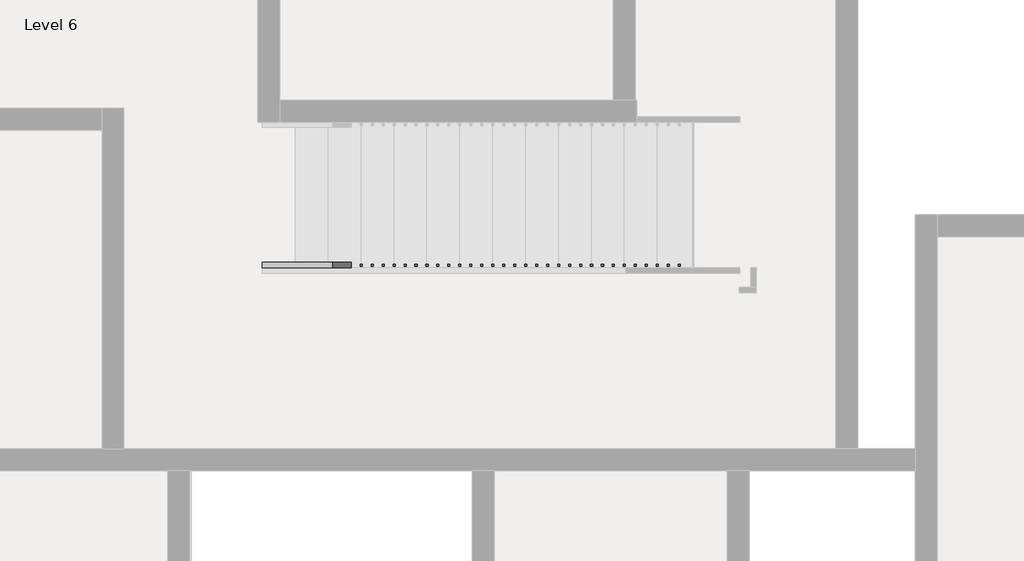
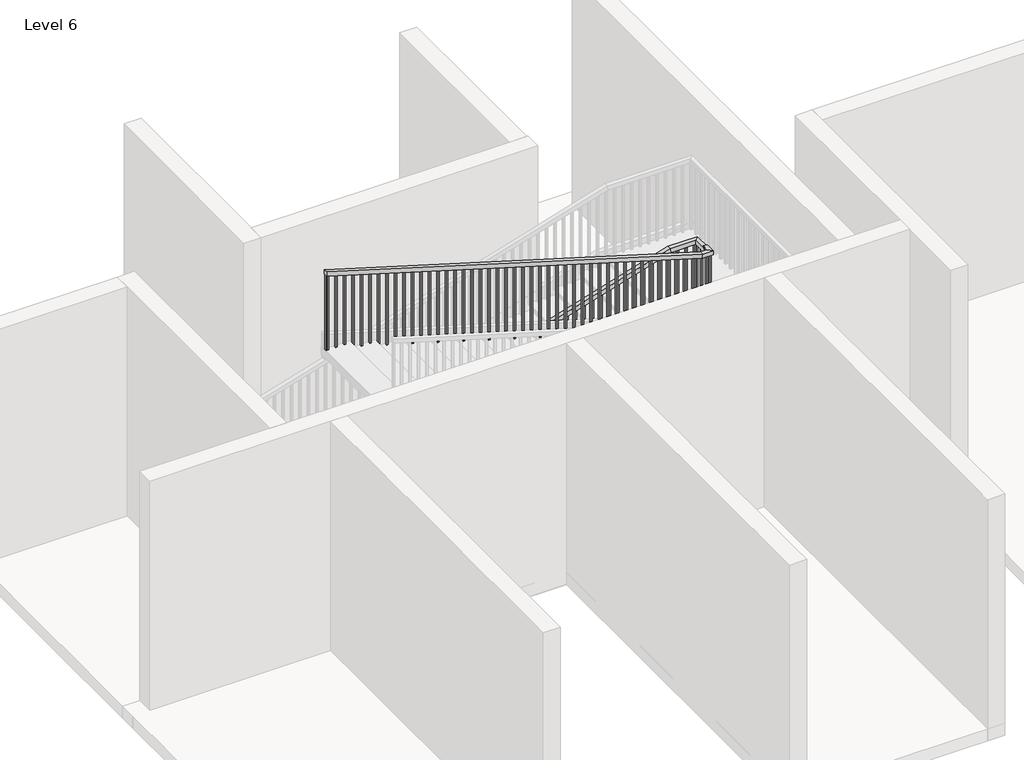
# One storey, part 11 of 14: 1 railing.
"""IFC4 building model written with IfcOpenShell, lengths in millimetres."""

from ifc_helpers import new_model, si_unit, frame, origin, place, context, project, spatial, polyline, outline, extrude, faceted_brep, element, save

model = new_model("IFC4")

# Units and contexts
model_context = context("Model", 3, world=origin())
ifc_project = project(units=[si_unit("LENGTHUNIT", "METRE", prefix="MILLI")], contexts=[model_context])

# Site, building, storey
site = spatial("IfcSite", under=ifc_project)
building = spatial("IfcBuilding", under=site)
storey = spatial("IfcBuildingStorey", under=building, Name="Level 6", Elevation=15240.0)

# Railing
placement = place(None, origin())
element("IfcRailing", 1, ObjectType="Handrail - Rectangular", at=placement, inside=storey, context=model_context, shape_type="SolidModel", body=[
    faceted_brep([(-5254.0891351, 11205.0082924, 16245.84), (-5254.0891351, 11205.0082924, 16192.8032429), (-5254.0891351, 11154.2082924, 16192.8032429), (-5254.0891351, 11154.2082924, 16245.84), (-986.8891351, 11205.0082924, 17526.0), (-979.4332782, 11205.0082924, 17475.2), (-979.4332782, 11154.2082924, 17475.2), (-986.8891351, 11154.2082924, 17526.0), (-631.2891351, 11205.0082924, 17526.0), (-631.2891351, 11205.0082924, 17475.2), (-682.0891351, 11154.2082924, 17475.2), (-682.0891351, 11154.2082924, 17526.0), (-631.2891351, 11001.8082924, 17526.0), (-631.2891351, 10951.0082924, 17475.2), (-682.0891351, 10951.0082924, 17475.2), (-682.0891351, 11001.8082924, 17526.0), (-631.2891351, 11001.8082924, 17548.86), (-631.2891351, 10951.0082924, 17498.06), (-682.0891351, 10951.0082924, 17498.06), (-682.0891351, 11001.8082924, 17548.86), (-631.2891351, 10874.8082924, 17548.86), (-631.2891351, 10874.8082924, 17498.06), (-682.0891351, 10925.6082924, 17498.06), (-682.0891351, 10925.6082924, 17548.86), (-758.2891351, 10874.8082924, 17548.86), (-765.744992, 10874.8082924, 17498.06), (-765.744992, 10925.6082924, 17498.06), (-758.2891351, 10925.6082924, 17548.86), (-5254.0891351, 10874.8082924, 18897.6), (-5254.0891351, 10925.6082924, 18897.6), (-5254.0891351, 10925.6082924, 18844.5632429), (-5254.0891351, 10874.8082924, 18844.5632429)], [[[0, 1, 2, 3]], [[1, 0, 4, 5]], [[2, 1, 5, 6]], [[3, 2, 6, 7]], [[0, 3, 7, 4]], [[5, 4, 8, 9]], [[6, 5, 9, 10]], [[7, 6, 10, 11]], [[4, 7, 11, 8]], [[9, 8, 12, 13]], [[10, 9, 13, 14]], [[11, 10, 14, 15]], [[8, 11, 15, 12]], [[13, 12, 16, 17]], [[14, 13, 17, 18]], [[15, 14, 18, 19]], [[12, 15, 19, 16]], [[17, 16, 20, 21]], [[18, 17, 21, 22]], [[19, 18, 22, 23]], [[16, 19, 23, 20]], [[21, 20, 24, 25]], [[22, 21, 25, 26]], [[23, 22, 26, 27]], [[20, 23, 27, 24]], [[28, 29, 30, 31]], [[25, 24, 28, 31]], [[26, 25, 31, 30]], [[27, 26, 30, 29]], [[24, 27, 29, 28]]]),
    extrude(outline(polyline([(18834.0857429, -5219.1641351), (18839.8007429, -5238.2141351), (17891.76, -5238.2141351), (17891.76, -5219.1641351), (18834.0857429, -5219.1641351)])), frame((0.0, 10890.6832924, 0.0), z_axis=(0.0, 1.0, 0.0), x_axis=(0.0, 0.0, 1.0)), (0.0, 0.0, 1.0), 19.05),
    extrude(outline(polyline([(18803.6057429, -5117.5641351), (18809.3207429, -5136.6141351), (17891.76, -5136.6141351), (17891.76, -5117.5641351), (18803.6057429, -5117.5641351)])), frame((0.0, 10890.6832924, 0.0), z_axis=(0.0, 1.0, 0.0), x_axis=(0.0, 0.0, 1.0)), (0.0, 0.0, 1.0), 19.05),
    extrude(outline(polyline([(18773.1257429, -5015.9641351), (18778.8407429, -5035.0141351), (17891.76, -5035.0141351), (17891.76, -5015.9641351), (18773.1257429, -5015.9641351)])), frame((0.0, 10890.6832924, 0.0), z_axis=(0.0, 1.0, 0.0), x_axis=(0.0, 0.0, 1.0)), (0.0, 0.0, 1.0), 19.05),
    extrude(outline(polyline([(18742.6457429, -4914.3641351), (18748.3607429, -4933.4141351), (17800.32, -4933.4141351), (17800.32, -4914.3641351), (18742.6457429, -4914.3641351)])), frame((0.0, 10890.6832924, 0.0), z_axis=(0.0, 1.0, 0.0), x_axis=(0.0, 0.0, 1.0)), (0.0, 0.0, 1.0), 19.05),
    extrude(outline(polyline([(18712.1657429, -4812.7641351), (18717.8807429, -4831.8141351), (17800.32, -4831.8141351), (17800.32, -4812.7641351), (18712.1657429, -4812.7641351)])), frame((0.0, 10890.6832924, 0.0), z_axis=(0.0, 1.0, 0.0), x_axis=(0.0, 0.0, 1.0)), (0.0, 0.0, 1.0), 19.05),
    extrude(outline(polyline([(18681.6857429, -4711.1641351), (18687.4007429, -4730.2141351), (17800.32, -4730.2141351), (17800.32, -4711.1641351), (18681.6857429, -4711.1641351)])), frame((0.0, 10890.6832924, 0.0), z_axis=(0.0, 1.0, 0.0), x_axis=(0.0, 0.0, 1.0)), (0.0, 0.0, 1.0), 19.05),
    extrude(outline(polyline([(18651.2057429, -4609.5641351), (18656.9207429, -4628.6141351), (17708.88, -4628.6141351), (17708.88, -4609.5641351), (18651.2057429, -4609.5641351)])), frame((0.0, 10890.6832924, 0.0), z_axis=(0.0, 1.0, 0.0), x_axis=(0.0, 0.0, 1.0)), (0.0, 0.0, 1.0), 19.05),
    extrude(outline(polyline([(18620.7257429, -4507.9641351), (18626.4407429, -4527.0141351), (17708.88, -4527.0141351), (17708.88, -4507.9641351), (18620.7257429, -4507.9641351)])), frame((0.0, 10890.6832924, 0.0), z_axis=(0.0, 1.0, 0.0), x_axis=(0.0, 0.0, 1.0)), (0.0, 0.0, 1.0), 19.05),
    extrude(outline(polyline([(18590.2457429, -4406.3641351), (18595.9607429, -4425.4141351), (17708.88, -4425.4141351), (17708.88, -4406.3641351), (18590.2457429, -4406.3641351)])), frame((0.0, 10890.6832924, 0.0), z_axis=(0.0, 1.0, 0.0), x_axis=(0.0, 0.0, 1.0)), (0.0, 0.0, 1.0), 19.05),
    extrude(outline(polyline([(18559.7657429, -4304.7641351), (18565.4807429, -4323.8141351), (17617.44, -4323.8141351), (17617.44, -4304.7641351), (18559.7657429, -4304.7641351)])), frame((0.0, 10890.6832924, 0.0), z_axis=(0.0, 1.0, 0.0), x_axis=(0.0, 0.0, 1.0)), (0.0, 0.0, 1.0), 19.05),
    extrude(outline(polyline([(18529.2857429, -4203.1641351), (18535.0007429, -4222.2141351), (17617.44, -4222.2141351), (17617.44, -4203.1641351), (18529.2857429, -4203.1641351)])), frame((0.0, 10890.6832924, 0.0), z_axis=(0.0, 1.0, 0.0), x_axis=(0.0, 0.0, 1.0)), (0.0, 0.0, 1.0), 19.05),
    extrude(outline(polyline([(18498.8057429, -4101.5641351), (18504.5207429, -4120.6141351), (17617.44, -4120.6141351), (17617.44, -4101.5641351), (18498.8057429, -4101.5641351)])), frame((0.0, 10890.6832924, 0.0), z_axis=(0.0, 1.0, 0.0), x_axis=(0.0, 0.0, 1.0)), (0.0, 0.0, 1.0), 19.05),
    extrude(outline(polyline([(18468.3257429, -3999.9641351), (18474.0407429, -4019.0141351), (17526.0, -4019.0141351), (17526.0, -3999.9641351), (18468.3257429, -3999.9641351)])), frame((0.0, 10890.6832924, 0.0), z_axis=(0.0, 1.0, 0.0), x_axis=(0.0, 0.0, 1.0)), (0.0, 0.0, 1.0), 19.05),
    extrude(outline(polyline([(18437.8457429, -3898.3641351), (18443.5607429, -3917.4141351), (17526.0, -3917.4141351), (17526.0, -3898.3641351), (18437.8457429, -3898.3641351)])), frame((0.0, 10890.6832924, 0.0), z_axis=(0.0, 1.0, 0.0), x_axis=(0.0, 0.0, 1.0)), (0.0, 0.0, 1.0), 19.05),
    extrude(outline(polyline([(18407.3657429, -3796.7641351), (18413.0807429, -3815.8141351), (17526.0, -3815.8141351), (17526.0, -3796.7641351), (18407.3657429, -3796.7641351)])), frame((0.0, 10890.6832924, 0.0), z_axis=(0.0, 1.0, 0.0), x_axis=(0.0, 0.0, 1.0)), (0.0, 0.0, 1.0), 19.05),
    extrude(outline(polyline([(18376.8857429, -3695.1641351), (18382.6007429, -3714.2141351), (17434.56, -3714.2141351), (17434.56, -3695.1641351), (18376.8857429, -3695.1641351)])), frame((0.0, 10890.6832924, 0.0), z_axis=(0.0, 1.0, 0.0), x_axis=(0.0, 0.0, 1.0)), (0.0, 0.0, 1.0), 19.05),
    extrude(outline(polyline([(18346.4057429, -3593.5641351), (18352.1207429, -3612.6141351), (17434.56, -3612.6141351), (17434.56, -3593.5641351), (18346.4057429, -3593.5641351)])), frame((0.0, 10890.6832924, 0.0), z_axis=(0.0, 1.0, 0.0), x_axis=(0.0, 0.0, 1.0)), (0.0, 0.0, 1.0), 19.05),
    extrude(outline(polyline([(18315.9257429, -3491.9641351), (18321.6407429, -3511.0141351), (17434.56, -3511.0141351), (17434.56, -3491.9641351), (18315.9257429, -3491.9641351)])), frame((0.0, 10890.6832924, 0.0), z_axis=(0.0, 1.0, 0.0), x_axis=(0.0, 0.0, 1.0)), (0.0, 0.0, 1.0), 19.05),
    extrude(outline(polyline([(18285.4457429, -3390.3641351), (18291.1607429, -3409.4141351), (17343.12, -3409.4141351), (17343.12, -3390.3641351), (18285.4457429, -3390.3641351)])), frame((0.0, 10890.6832924, 0.0), z_axis=(0.0, 1.0, 0.0), x_axis=(0.0, 0.0, 1.0)), (0.0, 0.0, 1.0), 19.05),
    extrude(outline(polyline([(18254.9657429, -3288.7641351), (18260.6807429, -3307.8141351), (17343.12, -3307.8141351), (17343.12, -3288.7641351), (18254.9657429, -3288.7641351)])), frame((0.0, 10890.6832924, 0.0), z_axis=(0.0, 1.0, 0.0), x_axis=(0.0, 0.0, 1.0)), (0.0, 0.0, 1.0), 19.05),
    extrude(outline(polyline([(18224.4857429, -3187.1641351), (18230.2007429, -3206.2141351), (17343.12, -3206.2141351), (17343.12, -3187.1641351), (18224.4857429, -3187.1641351)])), frame((0.0, 10890.6832924, 0.0), z_axis=(0.0, 1.0, 0.0), x_axis=(0.0, 0.0, 1.0)), (0.0, 0.0, 1.0), 19.05),
    extrude(outline(polyline([(18194.0057429, -3085.5641351), (18199.7207429, -3104.6141351), (17251.68, -3104.6141351), (17251.68, -3085.5641351), (18194.0057429, -3085.5641351)])), frame((0.0, 10890.6832924, 0.0), z_axis=(0.0, 1.0, 0.0), x_axis=(0.0, 0.0, 1.0)), (0.0, 0.0, 1.0), 19.05),
    extrude(outline(polyline([(18163.5257429, -2983.9641351), (18169.2407429, -3003.0141351), (17251.68, -3003.0141351), (17251.68, -2983.9641351), (18163.5257429, -2983.9641351)])), frame((0.0, 10890.6832924, 0.0), z_axis=(0.0, 1.0, 0.0), x_axis=(0.0, 0.0, 1.0)), (0.0, 0.0, 1.0), 19.05),
    extrude(outline(polyline([(18133.0457429, -2882.3641351), (18138.7607429, -2901.4141351), (17251.68, -2901.4141351), (17251.68, -2882.3641351), (18133.0457429, -2882.3641351)])), frame((0.0, 10890.6832924, 0.0), z_axis=(0.0, 1.0, 0.0), x_axis=(0.0, 0.0, 1.0)), (0.0, 0.0, 1.0), 19.05),
    extrude(outline(polyline([(18102.5657429, -2780.7641351), (18108.2807429, -2799.8141351), (17160.24, -2799.8141351), (17160.24, -2780.7641351), (18102.5657429, -2780.7641351)])), frame((0.0, 10890.6832924, 0.0), z_axis=(0.0, 1.0, 0.0), x_axis=(0.0, 0.0, 1.0)), (0.0, 0.0, 1.0), 19.05),
    extrude(outline(polyline([(18072.0857429, -2679.1641351), (18077.8007429, -2698.2141351), (17160.24, -2698.2141351), (17160.24, -2679.1641351), (18072.0857429, -2679.1641351)])), frame((0.0, 10890.6832924, 0.0), z_axis=(0.0, 1.0, 0.0), x_axis=(0.0, 0.0, 1.0)), (0.0, 0.0, 1.0), 19.05),
    extrude(outline(polyline([(18041.6057429, -2577.5641351), (18047.3207429, -2596.6141351), (17160.24, -2596.6141351), (17160.24, -2577.5641351), (18041.6057429, -2577.5641351)])), frame((0.0, 10890.6832924, 0.0), z_axis=(0.0, 1.0, 0.0), x_axis=(0.0, 0.0, 1.0)), (0.0, 0.0, 1.0), 19.05),
    extrude(outline(polyline([(18011.1257429, -2475.9641351), (18016.8407429, -2495.0141351), (17068.8, -2495.0141351), (17068.8, -2475.9641351), (18011.1257429, -2475.9641351)])), frame((0.0, 10890.6832924, 0.0), z_axis=(0.0, 1.0, 0.0), x_axis=(0.0, 0.0, 1.0)), (0.0, 0.0, 1.0), 19.05),
    extrude(outline(polyline([(17980.6457429, -2374.3641351), (17986.3607429, -2393.4141351), (17068.8, -2393.4141351), (17068.8, -2374.3641351), (17980.6457429, -2374.3641351)])), frame((0.0, 10890.6832924, 0.0), z_axis=(0.0, 1.0, 0.0), x_axis=(0.0, 0.0, 1.0)), (0.0, 0.0, 1.0), 19.05),
    extrude(outline(polyline([(17950.1657429, -2272.7641351), (17955.8807429, -2291.8141351), (17068.8, -2291.8141351), (17068.8, -2272.7641351), (17950.1657429, -2272.7641351)])), frame((0.0, 10890.6832924, 0.0), z_axis=(0.0, 1.0, 0.0), x_axis=(0.0, 0.0, 1.0)), (0.0, 0.0, 1.0), 19.05),
    extrude(outline(polyline([(17919.6857429, -2171.1641351), (17925.4007429, -2190.2141351), (16977.36, -2190.2141351), (16977.36, -2171.1641351), (17919.6857429, -2171.1641351)])), frame((0.0, 10890.6832924, 0.0), z_axis=(0.0, 1.0, 0.0), x_axis=(0.0, 0.0, 1.0)), (0.0, 0.0, 1.0), 19.05),
    extrude(outline(polyline([(17889.2057429, -2069.5641351), (17894.9207429, -2088.6141351), (16977.36, -2088.6141351), (16977.36, -2069.5641351), (17889.2057429, -2069.5641351)])), frame((0.0, 10890.6832924, 0.0), z_axis=(0.0, 1.0, 0.0), x_axis=(0.0, 0.0, 1.0)), (0.0, 0.0, 1.0), 19.05),
    extrude(outline(polyline([(17858.7257429, -1967.9641351), (17864.4407429, -1987.0141351), (16977.36, -1987.0141351), (16977.36, -1967.9641351), (17858.7257429, -1967.9641351)])), frame((0.0, 10890.6832924, 0.0), z_axis=(0.0, 1.0, 0.0), x_axis=(0.0, 0.0, 1.0)), (0.0, 0.0, 1.0), 19.05),
    extrude(outline(polyline([(17828.2457429, -1866.3641351), (17833.9607429, -1885.4141351), (16885.92, -1885.4141351), (16885.92, -1866.3641351), (17828.2457429, -1866.3641351)])), frame((0.0, 10890.6832924, 0.0), z_axis=(0.0, 1.0, 0.0), x_axis=(0.0, 0.0, 1.0)), (0.0, 0.0, 1.0), 19.05),
    extrude(outline(polyline([(17797.7657429, -1764.7641351), (17803.4807429, -1783.8141351), (16885.92, -1783.8141351), (16885.92, -1764.7641351), (17797.7657429, -1764.7641351)])), frame((0.0, 10890.6832924, 0.0), z_axis=(0.0, 1.0, 0.0), x_axis=(0.0, 0.0, 1.0)), (0.0, 0.0, 1.0), 19.05),
    extrude(outline(polyline([(17767.2857429, -1663.1641351), (17773.0007429, -1682.2141351), (16885.92, -1682.2141351), (16885.92, -1663.1641351), (17767.2857429, -1663.1641351)])), frame((0.0, 10890.6832924, 0.0), z_axis=(0.0, 1.0, 0.0), x_axis=(0.0, 0.0, 1.0)), (0.0, 0.0, 1.0), 19.05),
    extrude(outline(polyline([(17736.8057429, -1561.5641351), (17742.5207429, -1580.6141351), (16794.48, -1580.6141351), (16794.48, -1561.5641351), (17736.8057429, -1561.5641351)])), frame((0.0, 10890.6832924, 0.0), z_axis=(0.0, 1.0, 0.0), x_axis=(0.0, 0.0, 1.0)), (0.0, 0.0, 1.0), 19.05),
    extrude(outline(polyline([(17706.3257429, -1459.9641351), (17712.0407429, -1479.0141351), (16794.48, -1479.0141351), (16794.48, -1459.9641351), (17706.3257429, -1459.9641351)])), frame((0.0, 10890.6832924, 0.0), z_axis=(0.0, 1.0, 0.0), x_axis=(0.0, 0.0, 1.0)), (0.0, 0.0, 1.0), 19.05),
    extrude(outline(polyline([(17675.8457429, -1358.3641351), (17681.5607429, -1377.4141351), (16794.48, -1377.4141351), (16794.48, -1358.3641351), (17675.8457429, -1358.3641351)])), frame((0.0, 10890.6832924, 0.0), z_axis=(0.0, 1.0, 0.0), x_axis=(0.0, 0.0, 1.0)), (0.0, 0.0, 1.0), 19.05),
    extrude(outline(polyline([(17645.3657429, -1256.7641351), (17651.0807429, -1275.8141351), (16703.04, -1275.8141351), (16703.04, -1256.7641351), (17645.3657429, -1256.7641351)])), frame((0.0, 10890.6832924, 0.0), z_axis=(0.0, 1.0, 0.0), x_axis=(0.0, 0.0, 1.0)), (0.0, 0.0, 1.0), 19.05),
    extrude(outline(polyline([(17614.8857429, -1155.1641351), (17620.6007429, -1174.2141351), (16703.04, -1174.2141351), (16703.04, -1155.1641351), (17614.8857429, -1155.1641351)])), frame((0.0, 10890.6832924, 0.0), z_axis=(0.0, 1.0, 0.0), x_axis=(0.0, 0.0, 1.0)), (0.0, 0.0, 1.0), 19.05),
    extrude(outline(polyline([(17584.4057429, -1053.5641351), (17590.1207429, -1072.6141351), (16703.04, -1072.6141351), (16703.04, -1053.5641351), (17584.4057429, -1053.5641351)])), frame((0.0, 10890.6832924, 0.0), z_axis=(0.0, 1.0, 0.0), x_axis=(0.0, 0.0, 1.0)), (0.0, 0.0, 1.0), 19.05),
    extrude(outline(polyline([(17553.9257429, -951.9641351), (17559.6407429, -971.0141351), (16611.6, -971.0141351), (16611.6, -951.9641351), (17553.9257429, -951.9641351)])), frame((0.0, 10890.6832924, 0.0), z_axis=(0.0, 1.0, 0.0), x_axis=(0.0, 0.0, 1.0)), (0.0, 0.0, 1.0), 19.05),
    extrude(outline(polyline([(17523.4457429, -850.3641351), (17529.1607429, -869.4141351), (16611.6, -869.4141351), (16611.6, -850.3641351), (17523.4457429, -850.3641351)])), frame((0.0, 10890.6832924, 0.0), z_axis=(0.0, 1.0, 0.0), x_axis=(0.0, 0.0, 1.0)), (0.0, 0.0, 1.0), 19.05),
    extrude(outline(polyline([(17492.9657429, -748.7641351), (17498.6807429, -767.8141351), (16611.6, -767.8141351), (16611.6, -748.7641351), (17492.9657429, -748.7641351)])), frame((0.0, 10890.6832924, 0.0), z_axis=(0.0, 1.0, 0.0), x_axis=(0.0, 0.0, 1.0)), (0.0, 0.0, 1.0), 19.05),
    extrude(outline(polyline([(-666.2141351, 10985.9332924), (-647.1641351, 10985.9332924), (-647.1641351, 10966.8832924), (-666.2141351, 10966.8832924), (-666.2141351, 10985.9332924)])), frame((0.0, 0.0, 16611.6), z_axis=(0.0, 0.0, 1.0), x_axis=(1.0, 0.0, 0.0)), (0.0, 0.0, 1.0), 886.46),
    extrude(outline(polyline([(-666.2141351, 11087.5332924), (-647.1641351, 11087.5332924), (-647.1641351, 11068.4832924), (-666.2141351, 11068.4832924), (-666.2141351, 11087.5332924)])), frame((0.0, 0.0, 16611.6), z_axis=(0.0, 0.0, 1.0), x_axis=(1.0, 0.0, 0.0)), (0.0, 0.0, 1.0), 863.6),
    extrude(outline(polyline([(-691.6141351, 11170.0832924), (-691.6141351, 11189.1332924), (-672.5641351, 11189.1332924), (-672.5641351, 11170.0832924), (-691.6141351, 11170.0832924)])), frame((0.0, 0.0, 16611.6), z_axis=(0.0, 0.0, 1.0), x_axis=(1.0, 0.0, 0.0)), (0.0, 0.0, 1.0), 863.6),
    extrude(outline(polyline([(-793.2141351, 11170.0832924), (-793.2141351, 11189.1332924), (-774.1641351, 11189.1332924), (-774.1641351, 11170.0832924), (-793.2141351, 11170.0832924)])), frame((0.0, 0.0, 16611.6), z_axis=(0.0, 0.0, 1.0), x_axis=(1.0, 0.0, 0.0)), (0.0, 0.0, 1.0), 863.6),
    extrude(outline(polyline([(-894.8141351, 11170.0832924), (-894.8141351, 11189.1332924), (-875.7641351, 11189.1332924), (-875.7641351, 11170.0832924), (-894.8141351, 11170.0832924)])), frame((0.0, 0.0, 16611.6), z_axis=(0.0, 0.0, 1.0), x_axis=(1.0, 0.0, 0.0)), (0.0, 0.0, 1.0), 863.6),
    extrude(outline(polyline([(17475.8207429, -977.3641351), (17470.1057429, -996.4141351), (16611.6, -996.4141351), (16611.6, -977.3641351), (17475.8207429, -977.3641351)])), frame((0.0, 11170.0832924, 0.0), z_axis=(0.0, 1.0, 0.0), x_axis=(0.0, 0.0, 1.0)), (0.0, 0.0, 1.0), 19.05),
    extrude(outline(polyline([(17445.3407429, -1078.9641351), (17439.6257429, -1098.0141351), (16520.16, -1098.0141351), (16520.16, -1078.9641351), (17445.3407429, -1078.9641351)])), frame((0.0, 11170.0832924, 0.0), z_axis=(0.0, 1.0, 0.0), x_axis=(0.0, 0.0, 1.0)), (0.0, 0.0, 1.0), 19.05),
    extrude(outline(polyline([(17414.8607429, -1180.5641351), (17409.1457429, -1199.6141351), (16520.16, -1199.6141351), (16520.16, -1180.5641351), (17414.8607429, -1180.5641351)])), frame((0.0, 11170.0832924, 0.0), z_axis=(0.0, 1.0, 0.0), x_axis=(0.0, 0.0, 1.0)), (0.0, 0.0, 1.0), 19.05),
    extrude(outline(polyline([(17384.3807429, -1282.1641351), (17378.6657429, -1301.2141351), (16520.16, -1301.2141351), (16520.16, -1282.1641351), (17384.3807429, -1282.1641351)])), frame((0.0, 11170.0832924, 0.0), z_axis=(0.0, 1.0, 0.0), x_axis=(0.0, 0.0, 1.0)), (0.0, 0.0, 1.0), 19.05),
    extrude(outline(polyline([(17353.9007429, -1383.7641351), (17348.1857429, -1402.8141351), (16428.72, -1402.8141351), (16428.72, -1383.7641351), (17353.9007429, -1383.7641351)])), frame((0.0, 11170.0832924, 0.0), z_axis=(0.0, 1.0, 0.0), x_axis=(0.0, 0.0, 1.0)), (0.0, 0.0, 1.0), 19.05),
    extrude(outline(polyline([(17323.4207429, -1485.3641351), (17317.7057429, -1504.4141351), (16428.72, -1504.4141351), (16428.72, -1485.3641351), (17323.4207429, -1485.3641351)])), frame((0.0, 11170.0832924, 0.0), z_axis=(0.0, 1.0, 0.0), x_axis=(0.0, 0.0, 1.0)), (0.0, 0.0, 1.0), 19.05),
    extrude(outline(polyline([(17292.9407429, -1586.9641351), (17287.2257429, -1606.0141351), (16428.72, -1606.0141351), (16428.72, -1586.9641351), (17292.9407429, -1586.9641351)])), frame((0.0, 11170.0832924, 0.0), z_axis=(0.0, 1.0, 0.0), x_axis=(0.0, 0.0, 1.0)), (0.0, 0.0, 1.0), 19.05),
    extrude(outline(polyline([(17262.4607429, -1688.5641351), (17256.7457429, -1707.6141351), (16337.28, -1707.6141351), (16337.28, -1688.5641351), (17262.4607429, -1688.5641351)])), frame((0.0, 11170.0832924, 0.0), z_axis=(0.0, 1.0, 0.0), x_axis=(0.0, 0.0, 1.0)), (0.0, 0.0, 1.0), 19.05),
    extrude(outline(polyline([(17231.9807429, -1790.1641351), (17226.2657429, -1809.2141351), (16337.28, -1809.2141351), (16337.28, -1790.1641351), (17231.9807429, -1790.1641351)])), frame((0.0, 11170.0832924, 0.0), z_axis=(0.0, 1.0, 0.0), x_axis=(0.0, 0.0, 1.0)), (0.0, 0.0, 1.0), 19.05),
    extrude(outline(polyline([(17201.5007429, -1891.7641351), (17195.7857429, -1910.8141351), (16337.28, -1910.8141351), (16337.28, -1891.7641351), (17201.5007429, -1891.7641351)])), frame((0.0, 11170.0832924, 0.0), z_axis=(0.0, 1.0, 0.0), x_axis=(0.0, 0.0, 1.0)), (0.0, 0.0, 1.0), 19.05),
    extrude(outline(polyline([(17171.0207429, -1993.3641351), (17165.3057429, -2012.4141351), (16245.84, -2012.4141351), (16245.84, -1993.3641351), (17171.0207429, -1993.3641351)])), frame((0.0, 11170.0832924, 0.0), z_axis=(0.0, 1.0, 0.0), x_axis=(0.0, 0.0, 1.0)), (0.0, 0.0, 1.0), 19.05),
    extrude(outline(polyline([(17140.5407429, -2094.9641351), (17134.8257429, -2114.0141351), (16245.84, -2114.0141351), (16245.84, -2094.9641351), (17140.5407429, -2094.9641351)])), frame((0.0, 11170.0832924, 0.0), z_axis=(0.0, 1.0, 0.0), x_axis=(0.0, 0.0, 1.0)), (0.0, 0.0, 1.0), 19.05),
    extrude(outline(polyline([(17110.0607429, -2196.5641351), (17104.3457429, -2215.6141351), (16245.84, -2215.6141351), (16245.84, -2196.5641351), (17110.0607429, -2196.5641351)])), frame((0.0, 11170.0832924, 0.0), z_axis=(0.0, 1.0, 0.0), x_axis=(0.0, 0.0, 1.0)), (0.0, 0.0, 1.0), 19.05),
    extrude(outline(polyline([(17079.5807429, -2298.1641351), (17073.8657429, -2317.2141351), (16154.4, -2317.2141351), (16154.4, -2298.1641351), (17079.5807429, -2298.1641351)])), frame((0.0, 11170.0832924, 0.0), z_axis=(0.0, 1.0, 0.0), x_axis=(0.0, 0.0, 1.0)), (0.0, 0.0, 1.0), 19.05),
    extrude(outline(polyline([(17049.1007429, -2399.7641351), (17043.3857429, -2418.8141351), (16154.4, -2418.8141351), (16154.4, -2399.7641351), (17049.1007429, -2399.7641351)])), frame((0.0, 11170.0832924, 0.0), z_axis=(0.0, 1.0, 0.0), x_axis=(0.0, 0.0, 1.0)), (0.0, 0.0, 1.0), 19.05),
    extrude(outline(polyline([(17018.6207429, -2501.3641351), (17012.9057429, -2520.4141351), (16154.4, -2520.4141351), (16154.4, -2501.3641351), (17018.6207429, -2501.3641351)])), frame((0.0, 11170.0832924, 0.0), z_axis=(0.0, 1.0, 0.0), x_axis=(0.0, 0.0, 1.0)), (0.0, 0.0, 1.0), 19.05),
    extrude(outline(polyline([(16988.1407429, -2602.9641351), (16982.4257429, -2622.0141351), (16062.96, -2622.0141351), (16062.96, -2602.9641351), (16988.1407429, -2602.9641351)])), frame((0.0, 11170.0832924, 0.0), z_axis=(0.0, 1.0, 0.0), x_axis=(0.0, 0.0, 1.0)), (0.0, 0.0, 1.0), 19.05),
    extrude(outline(polyline([(16957.6607429, -2704.5641351), (16951.9457429, -2723.6141351), (16062.96, -2723.6141351), (16062.96, -2704.5641351), (16957.6607429, -2704.5641351)])), frame((0.0, 11170.0832924, 0.0), z_axis=(0.0, 1.0, 0.0), x_axis=(0.0, 0.0, 1.0)), (0.0, 0.0, 1.0), 19.05),
    extrude(outline(polyline([(16927.1807429, -2806.1641351), (16921.4657429, -2825.2141351), (16062.96, -2825.2141351), (16062.96, -2806.1641351), (16927.1807429, -2806.1641351)])), frame((0.0, 11170.0832924, 0.0), z_axis=(0.0, 1.0, 0.0), x_axis=(0.0, 0.0, 1.0)), (0.0, 0.0, 1.0), 19.05),
    extrude(outline(polyline([(16896.7007429, -2907.7641351), (16890.9857429, -2926.8141351), (15971.52, -2926.8141351), (15971.52, -2907.7641351), (16896.7007429, -2907.7641351)])), frame((0.0, 11170.0832924, 0.0), z_axis=(0.0, 1.0, 0.0), x_axis=(0.0, 0.0, 1.0)), (0.0, 0.0, 1.0), 19.05),
    extrude(outline(polyline([(16866.2207429, -3009.3641351), (16860.5057429, -3028.4141351), (15971.52, -3028.4141351), (15971.52, -3009.3641351), (16866.2207429, -3009.3641351)])), frame((0.0, 11170.0832924, 0.0), z_axis=(0.0, 1.0, 0.0), x_axis=(0.0, 0.0, 1.0)), (0.0, 0.0, 1.0), 19.05),
    extrude(outline(polyline([(16835.7407429, -3110.9641351), (16830.0257429, -3130.0141351), (15971.52, -3130.0141351), (15971.52, -3110.9641351), (16835.7407429, -3110.9641351)])), frame((0.0, 11170.0832924, 0.0), z_axis=(0.0, 1.0, 0.0), x_axis=(0.0, 0.0, 1.0)), (0.0, 0.0, 1.0), 19.05),
    extrude(outline(polyline([(16805.2607429, -3212.5641351), (16799.5457429, -3231.6141351), (15880.08, -3231.6141351), (15880.08, -3212.5641351), (16805.2607429, -3212.5641351)])), frame((0.0, 11170.0832924, 0.0), z_axis=(0.0, 1.0, 0.0), x_axis=(0.0, 0.0, 1.0)), (0.0, 0.0, 1.0), 19.05),
    extrude(outline(polyline([(16774.7807429, -3314.1641351), (16769.0657429, -3333.2141351), (15880.08, -3333.2141351), (15880.08, -3314.1641351), (16774.7807429, -3314.1641351)])), frame((0.0, 11170.0832924, 0.0), z_axis=(0.0, 1.0, 0.0), x_axis=(0.0, 0.0, 1.0)), (0.0, 0.0, 1.0), 19.05),
    extrude(outline(polyline([(16744.3007429, -3415.7641351), (16738.5857429, -3434.8141351), (15880.08, -3434.8141351), (15880.08, -3415.7641351), (16744.3007429, -3415.7641351)])), frame((0.0, 11170.0832924, 0.0), z_axis=(0.0, 1.0, 0.0), x_axis=(0.0, 0.0, 1.0)), (0.0, 0.0, 1.0), 19.05),
    extrude(outline(polyline([(16713.8207429, -3517.3641351), (16708.1057429, -3536.4141351), (15788.64, -3536.4141351), (15788.64, -3517.3641351), (16713.8207429, -3517.3641351)])), frame((0.0, 11170.0832924, 0.0), z_axis=(0.0, 1.0, 0.0), x_axis=(0.0, 0.0, 1.0)), (0.0, 0.0, 1.0), 19.05),
    extrude(outline(polyline([(16683.3407429, -3618.9641351), (16677.6257429, -3638.0141351), (15788.64, -3638.0141351), (15788.64, -3618.9641351), (16683.3407429, -3618.9641351)])), frame((0.0, 11170.0832924, 0.0), z_axis=(0.0, 1.0, 0.0), x_axis=(0.0, 0.0, 1.0)), (0.0, 0.0, 1.0), 19.05),
    extrude(outline(polyline([(16652.8607429, -3720.5641351), (16647.1457429, -3739.6141351), (15788.64, -3739.6141351), (15788.64, -3720.5641351), (16652.8607429, -3720.5641351)])), frame((0.0, 11170.0832924, 0.0), z_axis=(0.0, 1.0, 0.0), x_axis=(0.0, 0.0, 1.0)), (0.0, 0.0, 1.0), 19.05),
    extrude(outline(polyline([(16622.3807429, -3822.1641351), (16616.6657429, -3841.2141351), (15697.2, -3841.2141351), (15697.2, -3822.1641351), (16622.3807429, -3822.1641351)])), frame((0.0, 11170.0832924, 0.0), z_axis=(0.0, 1.0, 0.0), x_axis=(0.0, 0.0, 1.0)), (0.0, 0.0, 1.0), 19.05),
    extrude(outline(polyline([(16591.9007429, -3923.7641351), (16586.1857429, -3942.8141351), (15697.2, -3942.8141351), (15697.2, -3923.7641351), (16591.9007429, -3923.7641351)])), frame((0.0, 11170.0832924, 0.0), z_axis=(0.0, 1.0, 0.0), x_axis=(0.0, 0.0, 1.0)), (0.0, 0.0, 1.0), 19.05),
    extrude(outline(polyline([(16561.4207429, -4025.3641351), (16555.7057429, -4044.4141351), (15697.2, -4044.4141351), (15697.2, -4025.3641351), (16561.4207429, -4025.3641351)])), frame((0.0, 11170.0832924, 0.0), z_axis=(0.0, 1.0, 0.0), x_axis=(0.0, 0.0, 1.0)), (0.0, 0.0, 1.0), 19.05),
    extrude(outline(polyline([(16530.9407429, -4126.9641351), (16525.2257429, -4146.0141351), (15605.76, -4146.0141351), (15605.76, -4126.9641351), (16530.9407429, -4126.9641351)])), frame((0.0, 11170.0832924, 0.0), z_axis=(0.0, 1.0, 0.0), x_axis=(0.0, 0.0, 1.0)), (0.0, 0.0, 1.0), 19.05),
    extrude(outline(polyline([(16500.4607429, -4228.5641351), (16494.7457429, -4247.6141351), (15605.76, -4247.6141351), (15605.76, -4228.5641351), (16500.4607429, -4228.5641351)])), frame((0.0, 11170.0832924, 0.0), z_axis=(0.0, 1.0, 0.0), x_axis=(0.0, 0.0, 1.0)), (0.0, 0.0, 1.0), 19.05),
    extrude(outline(polyline([(16469.9807429, -4330.1641351), (16464.2657429, -4349.2141351), (15605.76, -4349.2141351), (15605.76, -4330.1641351), (16469.9807429, -4330.1641351)])), frame((0.0, 11170.0832924, 0.0), z_axis=(0.0, 1.0, 0.0), x_axis=(0.0, 0.0, 1.0)), (0.0, 0.0, 1.0), 19.05),
    extrude(outline(polyline([(16439.5007429, -4431.7641351), (16433.7857429, -4450.8141351), (15514.32, -4450.8141351), (15514.32, -4431.7641351), (16439.5007429, -4431.7641351)])), frame((0.0, 11170.0832924, 0.0), z_axis=(0.0, 1.0, 0.0), x_axis=(0.0, 0.0, 1.0)), (0.0, 0.0, 1.0), 19.05),
    extrude(outline(polyline([(16409.0207429, -4533.3641351), (16403.3057429, -4552.4141351), (15514.32, -4552.4141351), (15514.32, -4533.3641351), (16409.0207429, -4533.3641351)])), frame((0.0, 11170.0832924, 0.0), z_axis=(0.0, 1.0, 0.0), x_axis=(0.0, 0.0, 1.0)), (0.0, 0.0, 1.0), 19.05),
    extrude(outline(polyline([(16378.5407429, -4634.9641351), (16372.8257429, -4654.0141351), (15514.32, -4654.0141351), (15514.32, -4634.9641351), (16378.5407429, -4634.9641351)])), frame((0.0, 11170.0832924, 0.0), z_axis=(0.0, 1.0, 0.0), x_axis=(0.0, 0.0, 1.0)), (0.0, 0.0, 1.0), 19.05),
    extrude(outline(polyline([(16348.0607429, -4736.5641351), (16342.3457429, -4755.6141351), (15422.88, -4755.6141351), (15422.88, -4736.5641351), (16348.0607429, -4736.5641351)])), frame((0.0, 11170.0832924, 0.0), z_axis=(0.0, 1.0, 0.0), x_axis=(0.0, 0.0, 1.0)), (0.0, 0.0, 1.0), 19.05),
    extrude(outline(polyline([(16317.5807429, -4838.1641351), (16311.8657429, -4857.2141351), (15422.88, -4857.2141351), (15422.88, -4838.1641351), (16317.5807429, -4838.1641351)])), frame((0.0, 11170.0832924, 0.0), z_axis=(0.0, 1.0, 0.0), x_axis=(0.0, 0.0, 1.0)), (0.0, 0.0, 1.0), 19.05),
    extrude(outline(polyline([(16287.1007429, -4939.7641351), (16281.3857429, -4958.8141351), (15422.88, -4958.8141351), (15422.88, -4939.7641351), (16287.1007429, -4939.7641351)])), frame((0.0, 11170.0832924, 0.0), z_axis=(0.0, 1.0, 0.0), x_axis=(0.0, 0.0, 1.0)), (0.0, 0.0, 1.0), 19.05),
    extrude(outline(polyline([(16256.6207429, -5041.3641351), (16250.9057429, -5060.4141351), (15331.44, -5060.4141351), (15331.44, -5041.3641351), (16256.6207429, -5041.3641351)])), frame((0.0, 11170.0832924, 0.0), z_axis=(0.0, 1.0, 0.0), x_axis=(0.0, 0.0, 1.0)), (0.0, 0.0, 1.0), 19.05),
    extrude(outline(polyline([(16226.1407429, -5142.9641351), (16220.4257429, -5162.0141351), (15331.44, -5162.0141351), (15331.44, -5142.9641351), (16226.1407429, -5142.9641351)])), frame((0.0, 11170.0832924, 0.0), z_axis=(0.0, 1.0, 0.0), x_axis=(0.0, 0.0, 1.0)), (0.0, 0.0, 1.0), 19.05),
    extrude(outline(polyline([(-666.2141351, 10909.7332924), (-647.1641351, 10909.7332924), (-647.1641351, 10890.6832924), (-666.2141351, 10890.6832924), (-666.2141351, 10909.7332924)])), frame((0.0, 0.0, 16611.6), z_axis=(0.0, 0.0, 1.0), x_axis=(1.0, 0.0, 0.0)), (0.0, 0.0, 1.0), 886.46),
    extrude(outline(polyline([(-666.2141351, 11170.0832924), (-666.2141351, 11189.1332924), (-647.1641351, 11189.1332924), (-647.1641351, 11170.0832924), (-666.2141351, 11170.0832924)])), frame((0.0, 0.0, 16611.6), z_axis=(0.0, 0.0, 1.0), x_axis=(1.0, 0.0, 0.0)), (0.0, 0.0, 1.0), 863.6),
    extrude(outline(polyline([(18838.8482429, -5235.0391351), (18844.5632429, -5254.0891351), (17891.76, -5254.0891351), (17891.76, -5235.0391351), (18838.8482429, -5235.0391351)])), frame((0.0, 10890.6832924, 0.0), z_axis=(0.0, 1.0, 0.0), x_axis=(0.0, 0.0, 1.0)), (0.0, 0.0, 1.0), 19.05),
    extrude(outline(polyline([(16198.5182429, -5235.0391351), (16192.8032429, -5254.0891351), (15331.44, -5254.0891351), (15331.44, -5235.0391351), (16198.5182429, -5235.0391351)])), frame((0.0, 11170.0832924, 0.0), z_axis=(0.0, 1.0, 0.0), x_axis=(0.0, 0.0, 1.0)), (0.0, 0.0, 1.0), 19.05),
])

save(model, "model.ifc")

# Revit data of these elements
# Type "Handrail - Rectangular"
#   Assembly Code = "C2010400"
#   built-in parameter 1008612 = 0.0416667 (stored number, unit not read)
#   built-in parameter 1008611 = 0.0416667 (stored number, unit not read)
#   built-in parameter 1008609 = 0.333333 (stored number, unit not read)
#   built-in parameter 1008604 = 0.166667 (stored number, unit not read)
#   built-in parameter 1008603 = 0.166667 (stored number, unit not read)
#   Railing Height = 3' - 0"
#   built-in parameter 1008630 = 2
#   built-in parameter 1008610 = 2
#   built-in parameter 1008618 = Baluster - Square : 3/4"
# Element 1 (IfcRailing, "Handrail - Rectangular")
#   Phase Created = New Construction
